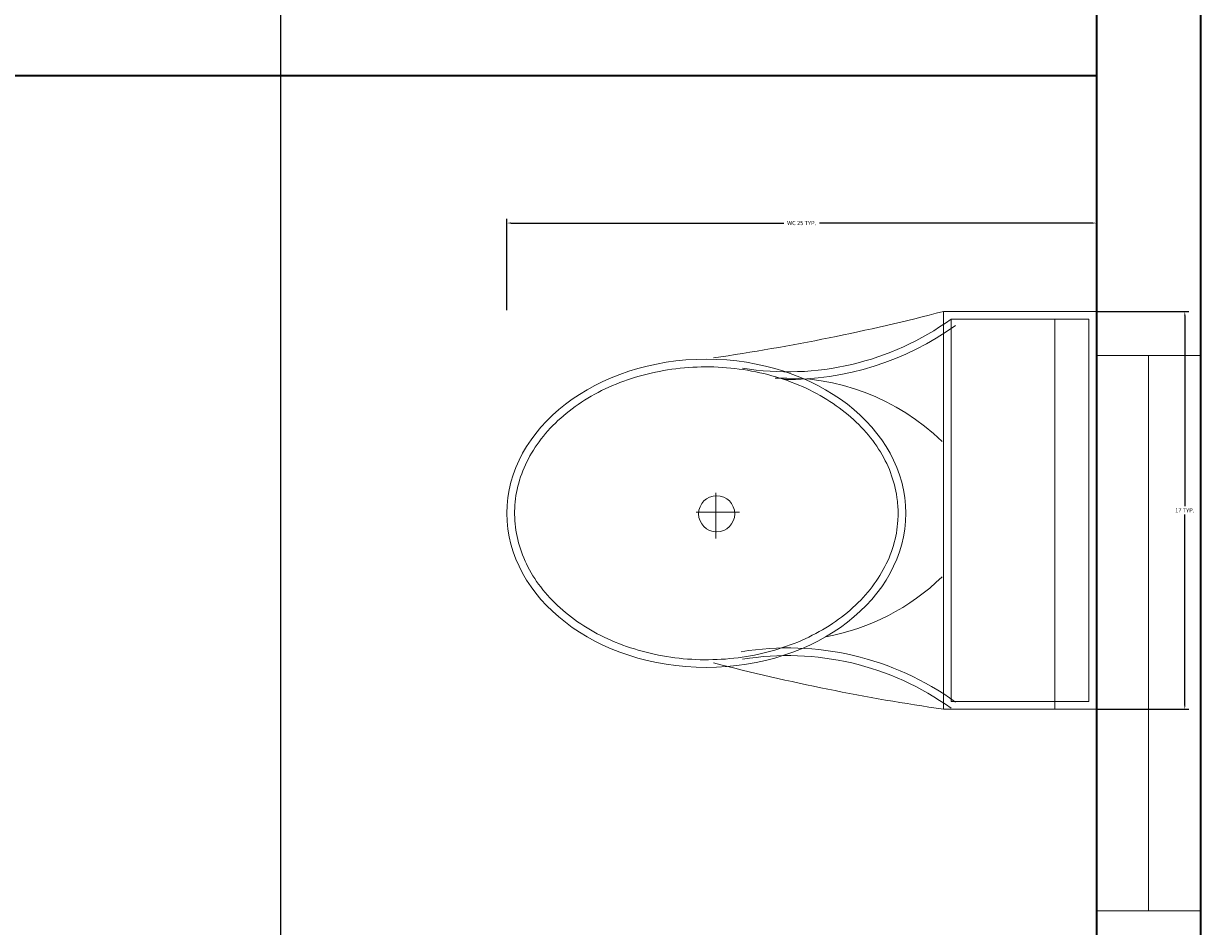
# Model space of a CAD drawing. Units: inches. Extents: x 1088 to 1703, y 668 to 1875.
# Tile 31 of 45: x 1539 to 1590, y 1567 to 1606. Entities that reach past the tile are written whole.
import ezdxf

# ---------------------------------------------------------------- set-up
doc = ezdxf.new("R2010")
doc.units = ezdxf.units.IN
for name, color, linetype, lineweight in [('A-ANNO-DIMS', 2, 'Continuous', 18), ('A-FLOR-FIXT', 8, 'Continuous', 18), ('A-GLAZ', 4, 'Continuous', 18), ('A-WALL', 7, 'Continuous', 35)]:
    doc.layers.add(name, color=color, linetype=linetype, lineweight=lineweight)
doc.styles.get("Standard").update_dxf_attribs({"font": 'arial.ttf'})
doc.dimstyles.get("Standard").update_dxf_attribs({"dimtxt": 0.18, "dimasz": 0.18, "dimexe": 0.18, "dimexo": 0.0625, "dimgap": 0.09, "dimtad": 0, "dimtih": 1, "dimtoh": 1, "dimdec": 4, "dimzin": 0, "dimdsep": 46, "dimtxsty": 'Standard', "dimcen": 0.09, "dimadec": 0, "dimazin": 0, "dimtfac": 1, "dimtdec": 4, "dimtofl": 0, "dimtmove": 0, "dimatfit": 3, "dimfxl": 1, "dimtolj": 1, "dimtzin": 0, "dimarcsym": 0})

# ---------------------------------------------------------------- blocks, each defined once
blk = doc.blocks.new('A$C31115884')
for p, q in [((257.5, 466.4), (257.5, 523.2)), ((283.1, 497.7), (223.4, 497.7)), ((0, 200), (0, 0)), ((520, 200), (0, 200)), ((10, 190), (10, 10)), ((510, 190), (10, 190)), ((510, 10), (510, 190)), ((520, 0), (520, 200)), ((510, 54.5), (0, 54.5)), ((10, 10), (510, 10)), ((0, 0), (520, 0))]:
    blk.add_line(p, q)
blk.add_circle((255.6, 496.4), 23.6)
for centre, radius, start, end in [((2777.7, -204.6), 2807, 165.4549, 171.7133), ((3237, 905), 2807, 188.2867, 194.5451), ((-294.5, 403.3), 364.7, 324.2091, 9.3499), ((-294.5, 403.3), 374.7, 324.2091, 9.3499), ((805.8, 403.3), 364.7, 170.6501, 215.7909), ((139.5, 406.2), 293.5, 315.8436, 2.6563), ((805.8, 403.3), 374.7, 179.2036, 215.7909), ((383.6, 406.2), 293.5, 190.2774, 224.1564)]:
    blk.add_arc(centre, radius, start, end)
blk.add_ellipse((256.2, 509.9), major_axis=(0, -260.7), ratio=0.772727)
blk.add_open_spline([(256.2, 259.2), (263.1, 259.2), (270, 259.7), (287.8, 262.3), (298.7, 265.1), (319.9, 273.1), (330.2, 278.4), (350.1, 291.1), (359.7, 298.7), (377.7, 315.9), (386.2, 325.5), (401.7, 346.6), (408.8, 358.1), (421.3, 382.5), (426.8, 395.5), (435.9, 422.4), (439.5, 436.4), (444.8, 465.1), (446.5, 479.7), (447.9, 509.2), (447.6, 524), (445, 553.3), (442.7, 567.8), (436.3, 596), (432.1, 609.7), (421.9, 636), (416, 648.6), (402.5, 672.1), (395, 683), (378.6, 703), (369.8, 712.1), (351.1, 728), (341.3, 734.8), (320.9, 746.2), (310.4, 750.7), (288.9, 757.3), (278, 759.4), (256, 761), (245, 760.6), (223.1, 757.2), (212.3, 754.3), (191.1, 746.1), (180.8, 740.7), (160.9, 727.8), (151.4, 720.1), (133.5, 702.7), (125.1, 693), (109.6, 671.7), (102.6, 660.2), (90.2, 635.7), (84.9, 622.7), (76, 595.6), (72.4, 581.6), (67.2, 552.9), (65.6, 538.2), (64.4, 508.8), (64.8, 494), (67.5, 464.7), (69.9, 450.2), (76.6, 422), (80.8, 408.3), (91.1, 382.2), (97.2, 369.7), (110.8, 346.3), (118.4, 335.4), (134.8, 315.6), (143.7, 306.7), (162.4, 290.9), (172.3, 284.2), (192.8, 273), (203.3, 268.6), (224.8, 262.2), (235.8, 260.2), (249.9, 259.3), (253, 259.2), (256.2, 259.2)], degree=3, knots=[0, 0, 0, 0, 0.110105, 0.110105, 0.285049, 0.285049, 0.459994, 0.459994, 0.634938, 0.634938, 0.809882, 0.809882, 0.984827, 0.984827, 1.159771, 1.159771, 1.334715, 1.334715, 1.50966, 1.50966, 1.684604, 1.684604, 1.859549, 1.859549, 2.034493, 2.034493, 2.209437, 2.209437, 2.384382, 2.384382, 2.559326, 2.559326, 2.73427, 2.73427, 2.909215, 2.909215, 3.084159, 3.084159, 3.259103, 3.259103, 3.434048, 3.434048, 3.608992, 3.608992, 3.783936, 3.783936, 3.958881, 3.958881, 4.133825, 4.133825, 4.30877, 4.30877, 4.483714, 4.483714, 4.658658, 4.658658, 4.833603, 4.833603, 5.008547, 5.008547, 5.183491, 5.183491, 5.358436, 5.358436, 5.53338, 5.53338, 5.708324, 5.708324, 5.883269, 5.883269, 6.058213, 6.058213, 6.233158, 6.233158, 6.283185, 6.283185, 6.283185, 6.283185])
blk = doc.blocks.new('WIN-24-OPPOSED-RETURN')
for p, q in [((0, 24), (4.5, 24)), ((4.5, 24), (2.25, 24)), ((2.25, 24), (2.25, 0)), ((2.25, 0), (0, 0)), ((0, 0), (4.5, 0))]:
    blk.add_line(p, q)
blk = doc.blocks.new('*D12')
at = {"layer": 'A-ANNO-DIMS', "color": 0, "lineweight": -2, "transparency": 16777216}
for p, q in [((1560.367, 1593.925), (1560.367, 1597.865)), ((1560.547, 1597.685), (1572.33, 1597.685)), ((1585.665, 1597.685), (1573.882, 1597.685)), ((1585.845, 1593.925), (1585.845, 1597.865))]:
    blk.add_line(p, q, dxfattribs=at)
at = {"layer": 'A-ANNO-DIMS', "color": 0, "transparency": 16777216}
for points in [[(1560.547, 1597.715), (1560.547, 1597.655), (1560.367, 1597.685)], [(1585.665, 1597.715), (1585.665, 1597.655), (1585.845, 1597.685)]]:
    blk.add_solid(points, dxfattribs=at)
at = {"layer": 'Defpoints', "color": 0, "transparency": 16777216}
for p in [(1560.367, 1597.685), (1560.367, 1593.863), (1585.845, 1593.863)]:
    blk.add_point(p, dxfattribs=at)
at = {"layer": 'A-ANNO-DIMS', "color": 0, "transparency": 16777216, "insert": (1573.106, 1597.685), "char_height": 0.18, "attachment_point": 5}
blk.add_mtext('\\A1;WC 25 TYP.', dxfattribs=at)
blk = doc.blocks.new('*D13')
at = {"layer": 'A-ANNO-DIMS', "color": 0, "lineweight": -2, "transparency": 16777216}
for p, q in [((1585.907, 1593.863), (1589.847, 1593.863)), ((1589.667, 1593.683), (1589.667, 1585.447)), ((1589.667, 1576.85), (1589.667, 1585.086)), ((1585.907, 1576.67), (1589.847, 1576.67))]:
    blk.add_line(p, q, dxfattribs=at)
at = {"layer": 'A-ANNO-DIMS', "color": 0, "transparency": 16777216}
for points in [[(1589.637, 1593.683), (1589.697, 1593.683), (1589.667, 1593.863)], [(1589.637, 1576.85), (1589.697, 1576.85), (1589.667, 1576.67)]]:
    blk.add_solid(points, dxfattribs=at)
at = {"layer": 'Defpoints', "color": 0, "transparency": 16777216}
for p in [(1585.845, 1593.863), (1589.667, 1593.863), (1585.845, 1576.67)]:
    blk.add_point(p, dxfattribs=at)
at = {"layer": 'A-ANNO-DIMS', "color": 0, "transparency": 16777216, "insert": (1589.667, 1585.266), "char_height": 0.18, "attachment_point": 5}
blk.add_mtext('\\A1;17 TYP.', dxfattribs=at)
blk = doc.blocks.new('*D32')
at = {"layer": 'A-ANNO-DIMS', "color": 0, "lineweight": -2, "transparency": 16777216}
for p, q in [((1550.595, 1373.121), (1550.595, 1857.788)), ((1550.775, 1857.608), (1567.825, 1857.608)), ((1585.665, 1857.608), (1568.614, 1857.608)), ((1585.845, 1360.983), (1585.845, 1857.788))]:
    blk.add_line(p, q, dxfattribs=at)
at = {"layer": 'A-ANNO-DIMS', "color": 0, "transparency": 16777216}
for points in [[(1550.775, 1857.638), (1550.775, 1857.578), (1550.595, 1857.608)], [(1585.665, 1857.638), (1585.665, 1857.578), (1585.845, 1857.608)]]:
    blk.add_solid(points, dxfattribs=at)
at = {"layer": 'Defpoints', "color": 0, "transparency": 16777216}
for p in [(1585.845, 1857.608), (1550.595, 1373.058), (1585.845, 1360.921)]:
    blk.add_point(p, dxfattribs=at)
at = {"layer": 'A-ANNO-DIMS', "color": 0, "transparency": 16777216, "insert": (1568.22, 1857.608), "char_height": 0.18, "attachment_point": 5}
blk.add_mtext('\\A1;35.25', dxfattribs=at)

msp = doc.modelspace()

# ---------------------------------------------------------------- linework, layer by layer
at = {"layer": 'A-WALL'}
for p, q in [((1590.345, 1673.058), (1590.345, 1539.558)), ((1585.845, 1668.558), (1585.845, 1544.058)), ((1489.845, 1604.058), (1585.845, 1604.058)), ((1585.845, 1604.058), (1585.845, 1544.058))]:
    msp.add_line(p, q, dxfattribs=at)

# ---------------------------------------------------------------- block references
at = {"layer": 'A-FLOR-FIXT', "xscale": 0.0330640103915726, "yscale": 0.0330640103915726, "zscale": 0.0330640103915726, "rotation": 89.99999999999996}
msp.add_blockref('A$C31115884', (1585.845, 1576.67), dxfattribs=at)
at = {"layer": 'A-GLAZ'}
msp.add_blockref('WIN-24-OPPOSED-RETURN', (1585.845, 1567.958), dxfattribs=at)

# ---------------------------------------------------------------- dimensions: what is measured, and where the dimension line sits
at = {"layer": 'A-ANNO-DIMS'}
dim = msp.add_linear_dim(base=(1585.845, 1857.608), p1=(1550.595, 1373.058), p2=(1585.845, 1360.921), dimstyle='Standard', override={"dimdec": 2, "dimlfac": 1, "dimrnd": 0, "dimzin": 0, "dimdsep": 46, "dimlunit": 2}, dxfattribs=at)
dim.commit()
dim.dimension.update_dxf_attribs({"geometry": '*D32', "text_midpoint": (1568.22, 1857.608)})
for base, p1, p2, angle, text, picture, middle in [((1560.367, 1597.685), (1585.845, 1593.863), (1560.367, 1593.863), 180, 'WC <> TYP.', '*D12', (1573.106, 1597.685)), ((1589.667, 1593.863), (1585.845, 1576.67), (1585.845, 1593.863), 90, '<> TYP.', '*D13', (1589.667, 1585.266))]:
    dim = msp.add_linear_dim(base=base, p1=p1, p2=p2, angle=angle, text=text, dimstyle='Standard', override={"dimdec": 0, "dimlfac": 1, "dimrnd": 0, "dimzin": 0, "dimdsep": 46, "dimlunit": 2}, dxfattribs=at)
    dim.commit()
    dim.dimension.update_dxf_attribs({"geometry": picture, "text_midpoint": middle})

doc.saveas('drawing.dxf')
